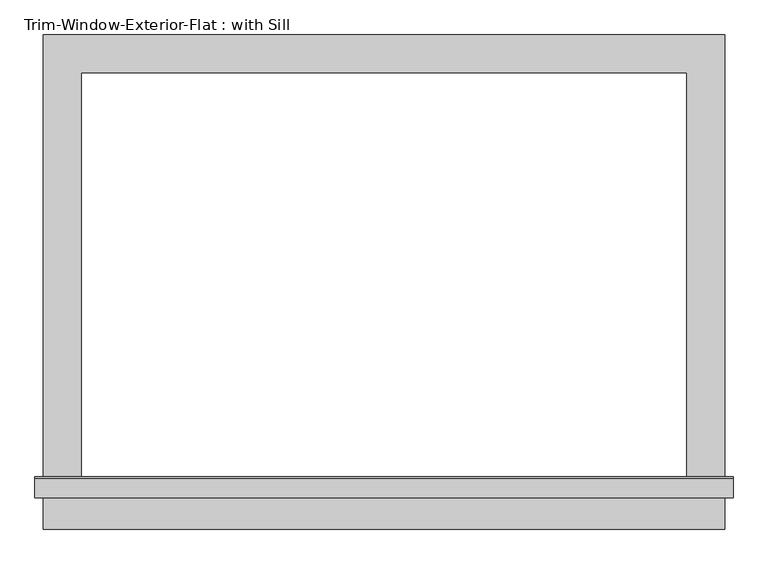
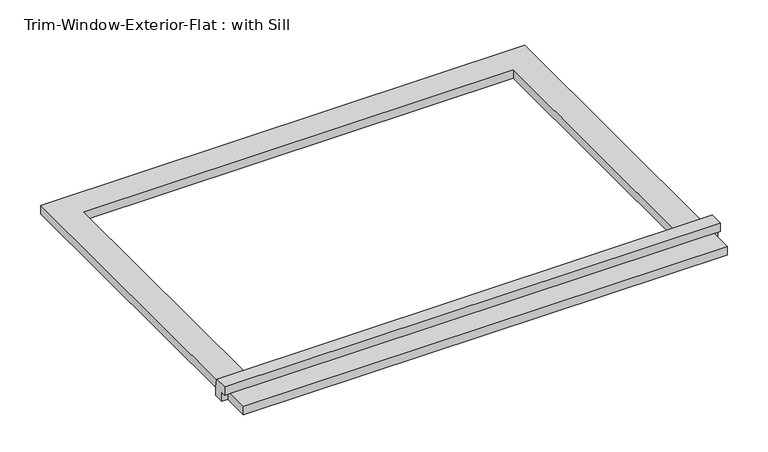
"""IFC4 building model written with IfcOpenShell, lengths in millimetres: proxy geometry, Trim-Window-Exterior-Flat : with Sill."""

from ifc_helpers import new_model, si_unit, frame, origin, origin_with_axes, place, context, project, spatial, polyline, outline, extrude, source, transform, mapped, element, save


def trim_window_exterior_flat_with_sill_40e754a6(model_context):
    return source(origin(), model_context, "Body", "SweptSolid", [
        extrude(outline(polyline([(514.35, -631.7823709), (514.35, -688.9323709), (-514.35, -688.9323709), (-514.35, -631.7823709), (514.35, -631.7823709)])), origin_with_axes(), (0.0, 0.0, 1.0), 19.05),
        extrude(outline(polyline([(-641.35, 38.1), (-612.0580645, 38.1), (-609.6, 19.05), (-609.6, 0.0), (-631.7823709, 0.0), (-631.7823709, 19.05), (-641.35, 19.05), (-641.35, 38.1)])), frame((-527.05, 0.0, 0.0), z_axis=(1.0, 0.0, 0.0), x_axis=(0.0, 1.0, 0.0)), (0.0, 0.0, 1.0), 1054.1),
        extrude(outline(polyline([(-514.35, 57.15), (514.35, 57.15), (514.35, -609.6), (457.2, -609.6), (457.2, 0.0), (-457.2, 0.0), (-457.2, -609.6), (-514.35, -609.6), (-514.35, 57.15)])), origin_with_axes(), (0.0, 0.0, 1.0), 19.05),
    ])


if __name__ == "__main__":
    model = new_model("IFC4")
    model_context = context("Model", 3, world=origin())
    ifc_project = project(units=[si_unit("LENGTHUNIT", "METRE", prefix="MILLI")], contexts=[model_context])
    site = spatial("IfcSite", under=ifc_project)
    building = spatial("IfcBuilding", under=site)
    placement = place(None, origin())
    trim_window_exterior_flat_with_sill_shape = trim_window_exterior_flat_with_sill_40e754a6(model_context)
    element("IfcBuildingElementProxy", 1, Name="Trim-Window-Exterior-Flat : with Sill", ObjectType="Trim-Window-Exterior-Flat : with Sill", at=placement, inside=building, context=model_context, shape_type="MappedRepresentation", body=[
        mapped(trim_window_exterior_flat_with_sill_shape, transform((0.0, 0.0, 0.0), x_axis=(1.0, 0.0, 0.0), y_axis=(0.0, 1.0, 0.0), z_axis=(0.0, 0.0, 1.0))),
    ])
    save(model, "model.ifc")

# Revit data of these elements
# Type "Trim-Window-Exterior-Flat : with Sill"
#   Trim Width = 0' - 2 1/4"
#   Trim Thickness_Picture Frame = 0' - 1 1/4"
#   Trim Thickness_with Sill = 0' - 0 3/4"
#   Sill Thickness = 0' - 1 1/4"
#   Opening Width [instance default] = 2' - 0"
#   Opening Height [instance default] = 3' - 0"
#   Default Elevation = 4' - 0"
#   Sill = yes
#   Picture Frame = no
#   Trim Material [instance default] = none
# Element 1 (IfcBuildingElementProxy, "Trim-Window-Exterior-Flat : with Sill")
#   Opening Width = 3' - 0"
#   Opening Height = 2' - 0"
#   Trim Material = Clad - White
#   Materials on its faces: "Clad - White"
# Materials
#   "Clad - White": class "Wood", colour RGB 0 0 0, transparency 0, Cost = 0
